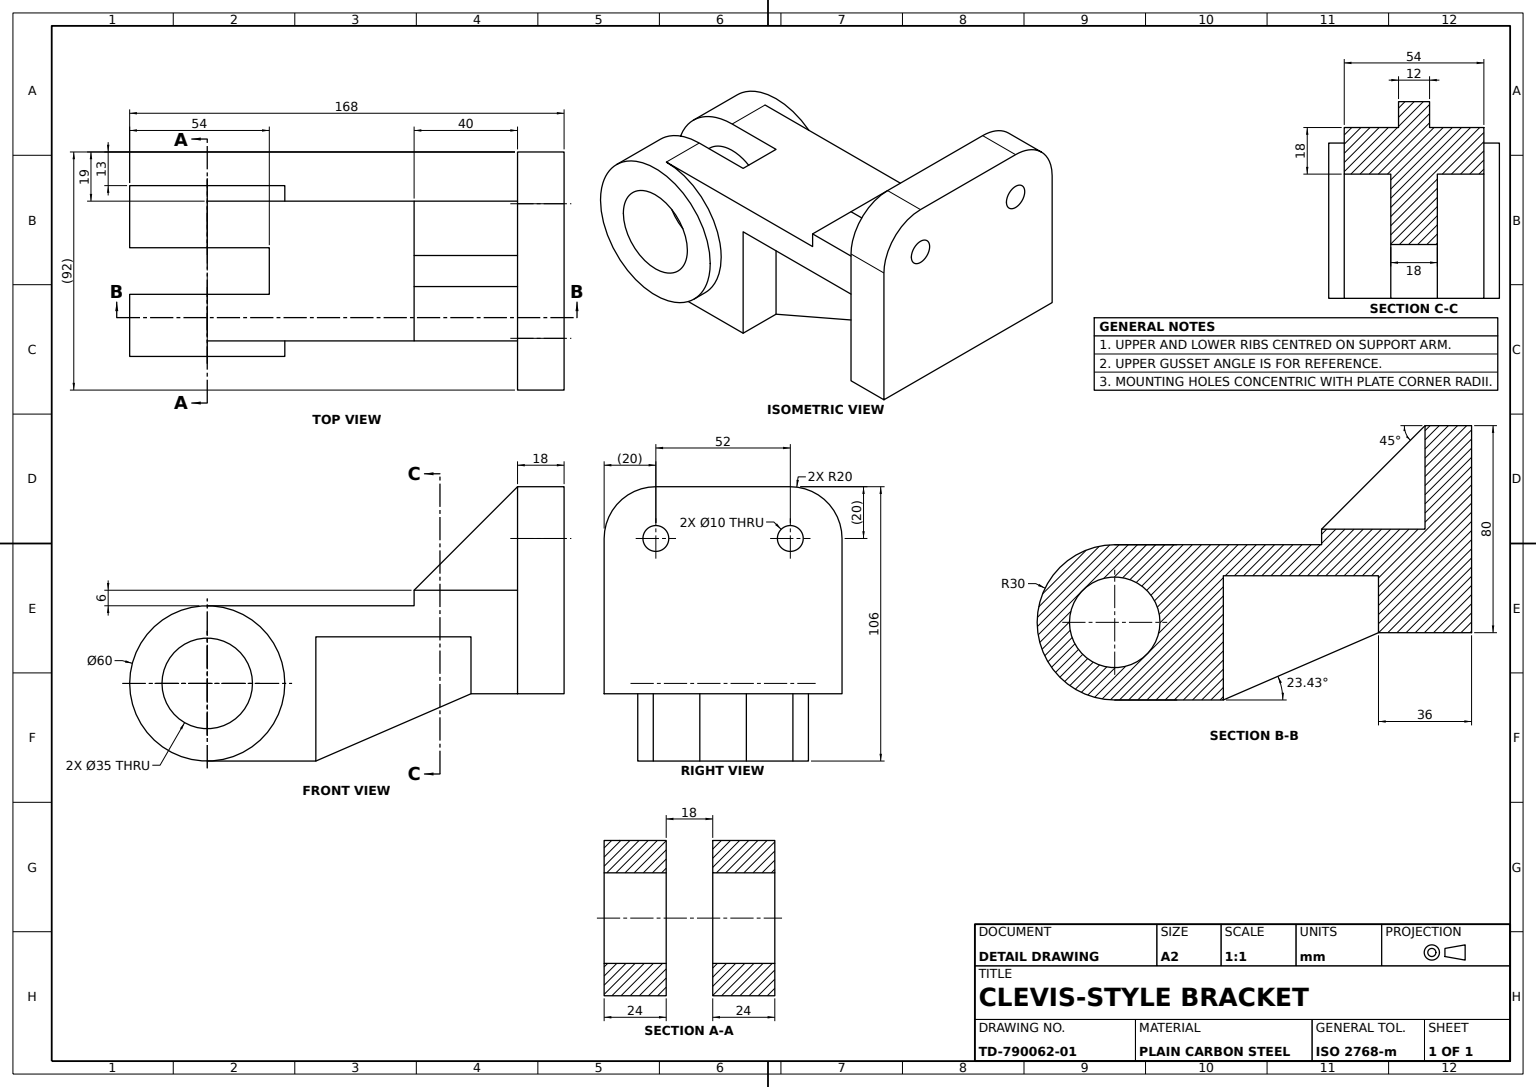
from build123d import *

# Parameters (mm, degrees)
HUB_PROFILE_R                = 30
HUB_PROFILE_R_2              = 17.5
BEARING_HUB_60_BORE_35_DEPTH = 33
SUPPORT_ARM_DEPTH            = 27
HUB_RIB_18_REACH             = 131.557
HUB_RIB_SKETCH_WALL_W        = 326.505005478
HUB_RIB_SKETCH_WALL_H        = 18
MOUNTING_PLATE_PROFILE_R     = 5
MOUNTING_PLATE_DEPTH         = 18
PLATE_RIB_12_REACH           = 166.122
PLATE_RIB_SKETCH_WALL_W      = 386.812354318
PLATE_RIB_SKETCH_WALL_H      = 12
FORK_SLOT_PROFILE_W          = 57.638691925
FORK_SLOT_PROFILE_H          = 18
FORK_SLOT_24X18_DEPTH        = 158.353106102


with BuildPart() as part:
    # Hub Profile → Bearing Hub Ø60 Bore Ø35 (new, symmetric)
    with BuildSketch(Plane.XY):
        Circle(HUB_PROFILE_R)
        Circle(HUB_PROFILE_R_2, mode=Mode.SUBTRACT)
    extrude(amount=BEARING_HUB_60_BORE_35_DEPTH, both=True)

    # Support Arm Profile → Support Arm (add, symmetric)
    with BuildSketch(Plane.XY):
        with BuildLine():
            Line((0, 30), (45.688517283, 30))
            Line((45.688517283, 30), (80, 30))
            Line((80, 30), (80, 36))
            Line((80, 36), (120, 36))
            Line((120, 36), (120, -4))
            Line((120, -4), (102, -4))
            Line((102, -4), (102, 18))
            Line((102, 18), (42, 18))
            Line((42, 18), (42, -30))
            Line((42, -30), (0, -30))
            ThreePointArc((0, -30), (30, 0), (0, 30))
        make_face()
    extrude(amount=SUPPORT_ARM_DEPTH, both=True)

    # Hub Rib Sketch wall → Hub Rib 18 (add, up to next)
    with BuildSketch(Plane(origin=(72, -17, 0), x_dir=(0.91755562531, 0.397607437634, 0), z_dir=(-0.397607437634, 0.91755562531, 0)), mode=Mode.PRIVATE) as hub_rib_18_sk1:
        Rectangle(HUB_RIB_SKETCH_WALL_W, HUB_RIB_SKETCH_WALL_H)
    hub_rib_18_tool1 = extrude(hub_rib_18_sk1.sketch, amount=HUB_RIB_18_REACH, mode=Mode.PRIVATE) - part.part
    add(hub_rib_18_tool1.solids().sort_by_distance((72, -17, 0))[0])

    # Mounting Plate Profile → Mounting Plate (add)
    with BuildSketch(Plane(origin=(120, 0, 0), x_dir=(0, 0, -1), z_dir=(1, 0, 0))):
        with BuildLine():
            Line((-46, -4), (46, -4))
            Line((46, -4), (46, 56))
            ThreePointArc((46, 56), (40.142135624, 70.142135624), (26, 76))
            Line((26, 76), (-26, 76))
            ThreePointArc((-26, 76), (-40.142135624, 70.142135624), (-46, 56))
            Line((-46, 56), (-46, -4))
        make_face()
        with Locations((-26, 56)):
            Circle(MOUNTING_PLATE_PROFILE_R, mode=Mode.SUBTRACT)
        with Locations((26, 56)):
            Circle(MOUNTING_PLATE_PROFILE_R, mode=Mode.SUBTRACT)
    extrude(amount=MOUNTING_PLATE_DEPTH)

    # Plate Rib Sketch wall → Plate Rib 12 (add, up to next)
    with BuildSketch(Plane(origin=(100, 56, 0), x_dir=(0.707106781187, 0.707106781187, 0), z_dir=(-0.707106781187, 0.707106781187, 0)), mode=Mode.PRIVATE) as plate_rib_12_sk1:
        Rectangle(PLATE_RIB_SKETCH_WALL_W, PLATE_RIB_SKETCH_WALL_H)
    plate_rib_12_tool1 = extrude(plate_rib_12_sk1.sketch, amount=-PLATE_RIB_12_REACH, mode=Mode.PRIVATE) - part.part
    add(plate_rib_12_tool1.solids().sort_by_distance((100, 56, 0))[0])

    # Fork Slot Profile → Fork Slot 24x18 (cut, through all)
    with BuildSketch(Plane(origin=(0, 30, 0), x_dir=(1, 0, 0), z_dir=(0, 1, 0))):
        with Locations((-4.819345963, 0)):
            Rectangle(FORK_SLOT_PROFILE_W, FORK_SLOT_PROFILE_H)
    extrude(amount=-FORK_SLOT_24X18_DEPTH, mode=Mode.SUBTRACT)


solid = part.part
